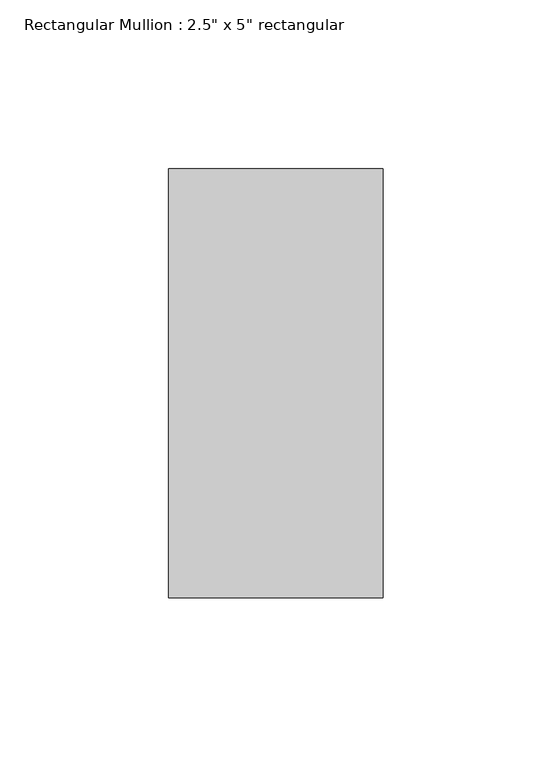
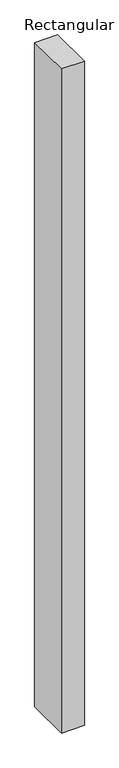
"""IFC4 building model written with IfcOpenShell, lengths in millimetres: member geometry."""

from ifc_helpers import new_model, si_unit, frame, origin, place, context, project, spatial, polyline, outline, extrude, source, transform, mapped, element, save


def member_e7372dc0(model_context):
    return source(origin(), model_context, "Body", "SweptSolid", [
        extrude(outline(polyline([(0.0, 63.5), (0.0, -63.5), (-63.5, -63.5), (-63.5, 63.5), (0.0, 63.5)])), frame((0.0, 0.0, -1934.6333333), z_axis=(0.0, 0.0, 1.0), x_axis=(1.0, 0.0, 0.0)), (0.0, 0.0, 1.0), 1934.6333333),
    ])


if __name__ == "__main__":
    model = new_model("IFC4")
    model_context = context("Model", 3, world=origin())
    ifc_project = project(units=[si_unit("LENGTHUNIT", "METRE", prefix="MILLI")], contexts=[model_context])
    site = spatial("IfcSite", under=ifc_project)
    building = spatial("IfcBuilding", under=site)
    placement = place(None, origin())
    member_shape = member_e7372dc0(model_context)
    element("IfcMember", 1, ObjectType="Rectangular Mullion : 2.5\" x 5\" rectangular", at=placement, inside=building, context=model_context, shape_type="MappedRepresentation", body=[
        mapped(member_shape, transform((0.0, 0.0, 0.0), x_axis=(1.0, 0.0, 0.0), y_axis=(0.0, 1.0, 0.0), z_axis=(0.0, 0.0, 1.0))),
    ])
    save(model, "model.ifc")

# Revit data of these elements
# Type "Rectangular Mullion : 2.5\" x 5\" rectangular"
#   built-in parameter 1007304 = 0.416667 (stored number, unit not read)
#   built-in parameter 1007301 = 0.104167 (stored number, unit not read)
#   built-in parameter 1007300 = 0.104167 (stored number, unit not read)
# Element 1 (IfcMember, "Rectangular Mullion : 2.5\" x 5\" rectangular")
#   Materials on its faces: "Aluminum"
# Materials
#   "Aluminum": class "Metal", colour RGB 247 247 247, transparency 0, Description = "Aluminum 6061", Cost = 0
